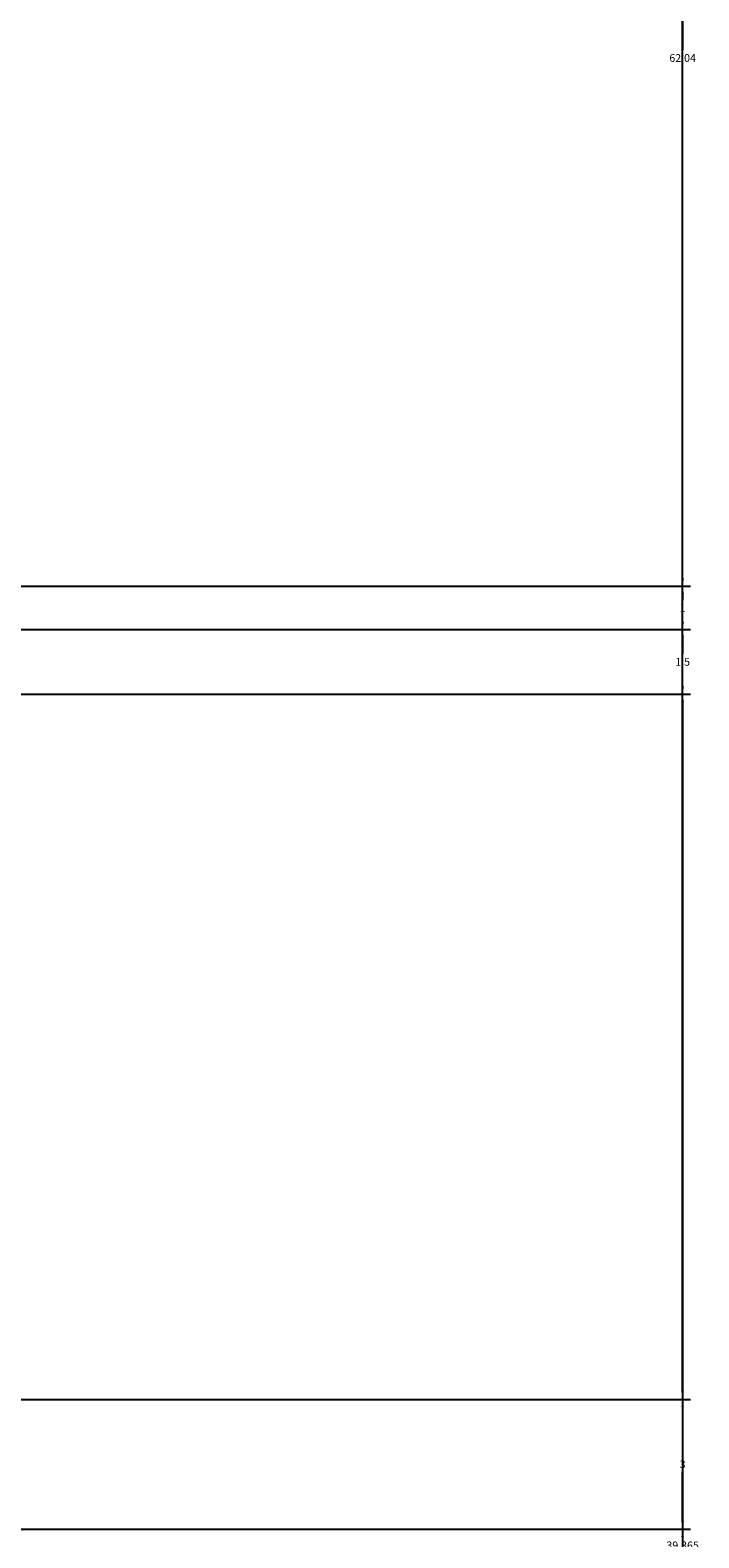
# Model space of a CAD drawing. Units: inches. Extents: x -6 to 289, y -8 to 323.
# Tile 74 of 107: x 273 to 289, y 159 to 194. Entities that reach past the tile are written whole.
import ezdxf

# ---------------------------------------------------------------- set-up
doc = ezdxf.new("R2010")
doc.units = ezdxf.units.IN
doc.header["$MEASUREMENT"] = 0
doc.layers.add('A-ANNO-DIMS', color=2, linetype='Continuous', lineweight=18)
doc.styles.get("Standard").update_dxf_attribs({"font": 'arial.ttf'})
doc.dimstyles.get("Standard").update_dxf_attribs({"dimtxt": 0.18, "dimasz": 0.18, "dimexe": 0.18, "dimexo": 0.0625, "dimgap": 0.09, "dimtad": 0, "dimtih": 1, "dimtoh": 1, "dimdec": 4, "dimzin": 0, "dimdsep": 46, "dimtxsty": 'Standard', "dimcen": 0.09, "dimadec": 0, "dimazin": 0, "dimtfac": 1, "dimtdec": 4, "dimtofl": 0, "dimtmove": 0, "dimatfit": 3, "dimfxl": 1, "dimtolj": 1, "dimtzin": 0, "dimarcsym": 0})

# ---------------------------------------------------------------- blocks, each defined once
blk = doc.blocks.new('*D24')
at = {"layer": 'A-ANNO-DIMS', "color": 0, "lineweight": -2, "transparency": 16777216}
for p, q in [((126.946, 178.654), (288.653, 178.654)), ((288.473, 178.474), (288.473, 159.153)), ((288.473, 139.469), (288.473, 158.789)), ((259.226, 139.289), (288.653, 139.289))]:
    blk.add_line(p, q, dxfattribs=at)
at = {"layer": 'A-ANNO-DIMS', "color": 0, "transparency": 16777216}
for points in [[(288.443, 178.474), (288.503, 178.474), (288.473, 178.654)], [(288.443, 139.469), (288.503, 139.469), (288.473, 139.289)]]:
    blk.add_solid(points, dxfattribs=at)
at = {"layer": 'Defpoints', "color": 0, "transparency": 16777216}
for p in [(126.883, 178.654), (288.473, 178.654), (259.164, 139.289)]:
    blk.add_point(p, dxfattribs=at)
at = {"layer": 'A-ANNO-DIMS', "color": 0, "transparency": 16777216, "insert": (288.473, 158.971), "char_height": 0.18, "attachment_point": 5}
blk.add_mtext('\\A1;39.365', dxfattribs=at)
blk = doc.blocks.new('*D25')
at = {"layer": 'A-ANNO-DIMS', "color": 0, "lineweight": -2, "transparency": 16777216}
for p, q in [((126.946, 226.654), (288.653, 226.654)), ((288.473, 226.474), (288.473, 202.836)), ((288.473, 178.834), (288.473, 202.472)), ((126.946, 178.654), (288.653, 178.654))]:
    blk.add_line(p, q, dxfattribs=at)
at = {"layer": 'A-ANNO-DIMS', "color": 0, "transparency": 16777216}
for points in [[(288.443, 226.474), (288.503, 226.474), (288.473, 226.654)], [(288.443, 178.834), (288.503, 178.834), (288.473, 178.654)]]:
    blk.add_solid(points, dxfattribs=at)
at = {"layer": 'Defpoints', "color": 0, "transparency": 16777216}
for p in [(126.883, 226.654), (288.473, 226.654), (126.883, 178.654)]:
    blk.add_point(p, dxfattribs=at)
at = {"layer": 'A-ANNO-DIMS', "color": 0, "transparency": 16777216, "insert": (288.473, 202.654), "char_height": 0.18, "attachment_point": 5}
blk.add_mtext('\\A1;48', dxfattribs=at)
blk = doc.blocks.new('*D35')
at = {"layer": 'A-ANNO-DIMS', "color": 0, "lineweight": -2, "transparency": 16777216}
for p, q in [((167.446, 180.154), (288.653, 180.154)), ((288.473, 179.974), (288.473, 179.586)), ((288.473, 178.834), (288.473, 179.222)), ((168.946, 178.654), (288.653, 178.654))]:
    blk.add_line(p, q, dxfattribs=at)
at = {"layer": 'A-ANNO-DIMS', "color": 0, "transparency": 16777216}
for points in [[(288.443, 179.974), (288.503, 179.974), (288.473, 180.154)], [(288.443, 178.834), (288.503, 178.834), (288.473, 178.654)]]:
    blk.add_solid(points, dxfattribs=at)
at = {"layer": 'Defpoints', "color": 0, "transparency": 16777216}
for p in [(167.383, 180.154), (288.473, 180.154), (168.883, 178.654)]:
    blk.add_point(p, dxfattribs=at)
at = {"layer": 'A-ANNO-DIMS', "color": 0, "transparency": 16777216, "insert": (288.473, 179.404), "char_height": 0.18, "attachment_point": 5}
blk.add_mtext('\\A1;1.5', dxfattribs=at)
blk = doc.blocks.new('*D36')
at = {"layer": 'A-ANNO-DIMS', "color": 0, "lineweight": -2, "transparency": 16777216}
for p, q in [((166.446, 181.154), (288.653, 181.154)), ((288.473, 180.974), (288.473, 180.834)), ((288.473, 180.334), (288.473, 180.474)), ((167.446, 180.154), (288.653, 180.154))]:
    blk.add_line(p, q, dxfattribs=at)
at = {"layer": 'A-ANNO-DIMS', "color": 0, "transparency": 16777216}
for points in [[(288.443, 180.974), (288.503, 180.974), (288.473, 181.154)], [(288.443, 180.334), (288.503, 180.334), (288.473, 180.154)]]:
    blk.add_solid(points, dxfattribs=at)
at = {"layer": 'Defpoints', "color": 0, "transparency": 16777216}
for p in [(166.383, 181.154), (288.473, 181.154), (167.383, 180.154)]:
    blk.add_point(p, dxfattribs=at)
at = {"layer": 'A-ANNO-DIMS', "color": 0, "transparency": 16777216, "insert": (288.473, 180.654), "char_height": 0.18, "attachment_point": 5}
blk.add_mtext('\\A1;1', dxfattribs=at)
blk = doc.blocks.new('*D37')
at = {"layer": 'A-ANNO-DIMS', "color": 0, "lineweight": -2, "transparency": 16777216}
for p, q in [((166.446, 224.154), (288.653, 224.154)), ((288.473, 223.974), (288.473, 202.836)), ((288.473, 181.334), (288.473, 202.472)), ((166.446, 181.154), (288.653, 181.154))]:
    blk.add_line(p, q, dxfattribs=at)
at = {"layer": 'A-ANNO-DIMS', "color": 0, "transparency": 16777216}
for points in [[(288.443, 223.974), (288.503, 223.974), (288.473, 224.154)], [(288.443, 181.334), (288.503, 181.334), (288.473, 181.154)]]:
    blk.add_solid(points, dxfattribs=at)
at = {"layer": 'Defpoints', "color": 0, "transparency": 16777216}
for p in [(166.383, 224.154), (288.473, 224.154), (166.383, 181.154)]:
    blk.add_point(p, dxfattribs=at)
at = {"layer": 'A-ANNO-DIMS', "color": 0, "transparency": 16777216, "insert": (288.473, 202.654), "char_height": 0.18, "attachment_point": 5}
blk.add_mtext('\\A1;43', dxfattribs=at)
blk = doc.blocks.new('*D47')
at = {"layer": 'A-ANNO-DIMS', "color": 0, "lineweight": -2, "transparency": 16777216}
for p, q in [((233.854, 224.389), (288.653, 224.389)), ((288.473, 224.209), (288.473, 193.55)), ((288.473, 162.528), (288.473, 193.187)), ((236.354, 162.348), (288.653, 162.348))]:
    blk.add_line(p, q, dxfattribs=at)
at = {"layer": 'A-ANNO-DIMS', "color": 0, "transparency": 16777216}
for points in [[(288.443, 224.209), (288.503, 224.209), (288.473, 224.389)], [(288.443, 162.528), (288.503, 162.528), (288.473, 162.348)]]:
    blk.add_solid(points, dxfattribs=at)
at = {"layer": 'Defpoints', "color": 0, "transparency": 16777216}
for p in [(233.792, 224.389), (288.473, 224.389), (236.292, 162.348)]:
    blk.add_point(p, dxfattribs=at)
at = {"layer": 'A-ANNO-DIMS', "color": 0, "transparency": 16777216, "insert": (288.473, 193.369), "char_height": 0.18, "attachment_point": 5}
blk.add_mtext('\\A1;62.04', dxfattribs=at)
blk = doc.blocks.new('*D103')
at = {"layer": 'A-ANNO-DIMS', "color": 0, "lineweight": -2, "transparency": 16777216}
for p, q in [((244.226, 159.348), (288.653, 159.348)), ((288.473, 159.168), (288.473, 151)), ((288.473, 142.469), (288.473, 150.637)), ((244.226, 142.289), (288.653, 142.289))]:
    blk.add_line(p, q, dxfattribs=at)
at = {"layer": 'A-ANNO-DIMS', "color": 0, "transparency": 16777216}
for points in [[(288.443, 159.168), (288.503, 159.168), (288.473, 159.348)], [(288.443, 142.469), (288.503, 142.469), (288.473, 142.289)]]:
    blk.add_solid(points, dxfattribs=at)
at = {"layer": 'Defpoints', "color": 0, "transparency": 16777216}
for p in [(244.164, 159.348), (288.473, 159.348), (244.164, 142.289)]:
    blk.add_point(p, dxfattribs=at)
at = {"layer": 'A-ANNO-DIMS', "color": 0, "transparency": 16777216, "insert": (288.473, 150.819), "char_height": 0.18, "attachment_point": 5}
blk.add_mtext('\\A1;17.06', dxfattribs=at)
blk = doc.blocks.new('*D104')
at = {"layer": 'A-ANNO-DIMS', "color": 0, "lineweight": -2, "transparency": 16777216}
for p, q in [((247.226, 162.348), (288.653, 162.348)), ((288.473, 162.168), (288.473, 161.03)), ((288.473, 159.528), (288.473, 160.666)), ((244.226, 159.348), (288.653, 159.348))]:
    blk.add_line(p, q, dxfattribs=at)
at = {"layer": 'A-ANNO-DIMS', "color": 0, "transparency": 16777216}
for points in [[(288.443, 162.168), (288.503, 162.168), (288.473, 162.348)], [(288.443, 159.528), (288.503, 159.528), (288.473, 159.348)]]:
    blk.add_solid(points, dxfattribs=at)
at = {"layer": 'Defpoints', "color": 0, "transparency": 16777216}
for p in [(247.164, 162.348), (288.473, 162.348), (244.164, 159.348)]:
    blk.add_point(p, dxfattribs=at)
at = {"layer": 'A-ANNO-DIMS', "color": 0, "transparency": 16777216, "insert": (288.473, 160.848), "char_height": 0.18, "attachment_point": 5}
blk.add_mtext('\\A1;3', dxfattribs=at)

msp = doc.modelspace()

# ---------------------------------------------------------------- dimensions: what is measured, and where the dimension line sits
at = {"layer": 'A-ANNO-DIMS'}
for base, p1, p2, override, picture, middle in [((288.4733, 226.654), (126.8835, 178.654), (126.8835, 226.654), {"dimdec": 0, "dimlfac": 1, "dimrnd": 0, "dimzin": 0, "dimdsep": 46, "dimlunit": 2}, '*D25', (288.4733, 202.654)), ((288.4733, 224.3887), (236.2918, 162.3484), (233.7918, 224.3887), {"dimdec": 2, "dimlfac": 1, "dimrnd": 0, "dimzin": 0, "dimdsep": 46, "dimlunit": 2}, '*D47', (288.4733, 193.3685)), ((288.4733, 224.154), (166.3835, 181.154), (166.3835, 224.154), {"dimdec": 0, "dimlfac": 1, "dimrnd": 0, "dimzin": 0, "dimdsep": 46, "dimlunit": 2}, '*D37', (288.4733, 202.654)), ((288.4733, 181.154), (167.3835, 180.154), (166.3835, 181.154), {"dimdec": 0, "dimlfac": 1, "dimrnd": 0, "dimzin": 0, "dimdsep": 46, "dimlunit": 2}, '*D36', (288.4733, 180.654)), ((288.4733, 180.154), (168.8835, 178.654), (167.3835, 180.154), {"dimdec": 1, "dimlfac": 1, "dimrnd": 0, "dimzin": 0, "dimdsep": 46, "dimlunit": 2}, '*D35', (288.4733, 179.404)), ((288.4733, 178.654), (259.1638, 139.2888), (126.8835, 178.654), {"dimdec": 3, "dimlfac": 1, "dimrnd": 0, "dimzin": 0, "dimdsep": 46, "dimlunit": 2}, '*D24', (288.4733, 158.9714)), ((288.4733, 162.3484), (244.1638, 159.3484), (247.1638, 162.3484), {"dimdec": 0, "dimlfac": 1, "dimrnd": 0, "dimzin": 0, "dimdsep": 46, "dimlunit": 2}, '*D104', (288.4733, 160.8484)), ((288.4733, 159.3484), (244.1638, 142.2888), (244.1638, 159.3484), {"dimdec": 2, "dimlfac": 1, "dimrnd": 0, "dimzin": 0, "dimdsep": 46, "dimlunit": 2}, '*D103', (288.4733, 150.8186))]:
    dim = msp.add_linear_dim(base=base, p1=p1, p2=p2, angle=90, dimstyle='Standard', override=override, dxfattribs=at)
    dim.commit()
    dim.dimension.update_dxf_attribs({"geometry": picture, "text_midpoint": middle})

doc.saveas('drawing.dxf')
